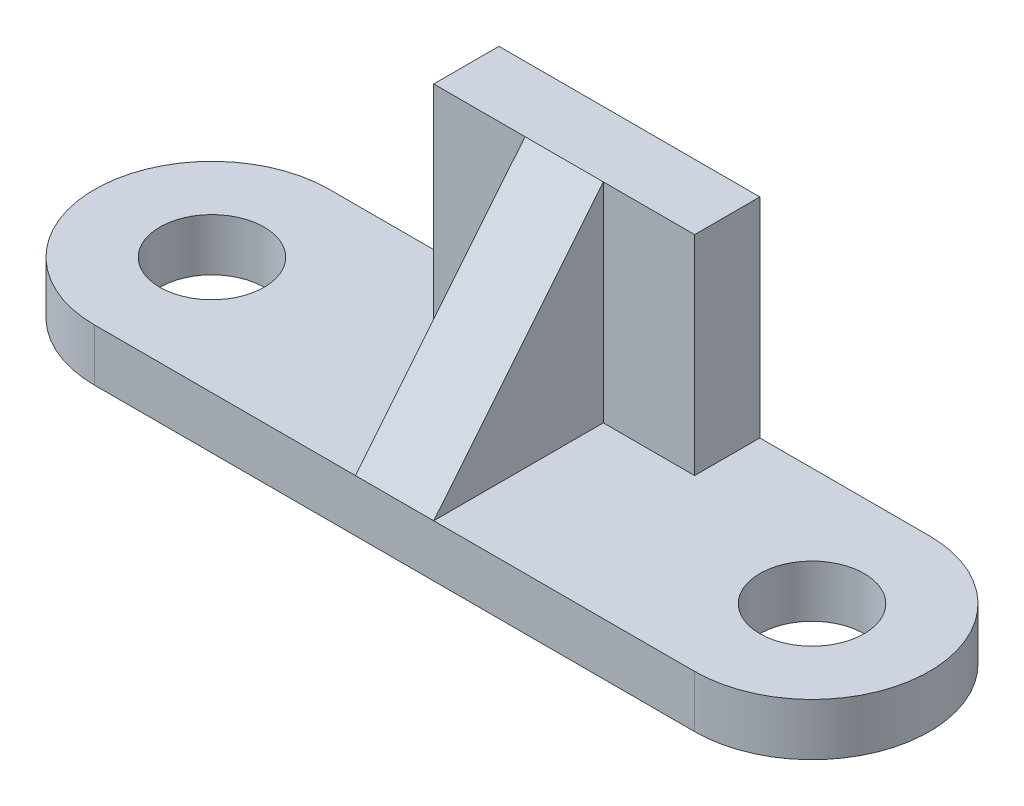
ISO-10303-21;
HEADER;
FILE_DESCRIPTION(('STEP AP214'),'2;1');
FILE_NAME('part.step','',(''),(''),'','','');
FILE_SCHEMA(('AUTOMOTIVE_DESIGN { 1 0 10303 214 1 1 1 1 }'));
ENDSEC;
DATA;
#1=APPLICATION_CONTEXT('core data for automotive mechanical design processes');
#2=APPLICATION_PROTOCOL_DEFINITION('international standard','automotive_design',2000,#1);
#3=PRODUCT_CONTEXT('',#1,'mechanical');
#4=PRODUCT('Part','Part','',(#3));
#5=PRODUCT_RELATED_PRODUCT_CATEGORY('part','',(#4));
#6=PRODUCT_DEFINITION_FORMATION('','',#4);
#7=PRODUCT_DEFINITION_CONTEXT('part definition',#1,'design');
#8=PRODUCT_DEFINITION('design','',#6,#7);
#9=PRODUCT_DEFINITION_SHAPE('','',#8);
#10=(LENGTH_UNIT() NAMED_UNIT(*) SI_UNIT(.MILLI.,.METRE.));
#11=(NAMED_UNIT(*) PLANE_ANGLE_UNIT() SI_UNIT($,.RADIAN.));
#12=(NAMED_UNIT(*) SI_UNIT($,.STERADIAN.) SOLID_ANGLE_UNIT());
#13=UNCERTAINTY_MEASURE_WITH_UNIT(LENGTH_MEASURE(1.E-05),#10,'distance_accuracy_value','');
#14=(GEOMETRIC_REPRESENTATION_CONTEXT(3) GLOBAL_UNCERTAINTY_ASSIGNED_CONTEXT((#13)) GLOBAL_UNIT_ASSIGNED_CONTEXT((#10,
#11,#12)) REPRESENTATION_CONTEXT('',''));
#15=CARTESIAN_POINT('',(0.,0.,0.));
#16=DIRECTION('',(0.,0.,1.));
#17=DIRECTION('',(1.,0.,0.));
#18=AXIS2_PLACEMENT_3D('',#15,#16,#17);
#19=CARTESIAN_POINT('',(-46.,8.,0.));
#20=DIRECTION('',(0.,1.,0.));
#21=DIRECTION('',(0.,0.,1.));
#22=AXIS2_PLACEMENT_3D('',#19,#20,#21);
#23=PLANE('',#22);
#24=CARTESIAN_POINT('',(-46.,8.,0.));
#25=DIRECTION('',(0.,1.,0.));
#26=DIRECTION('',(0.,0.,1.));
#27=AXIS2_PLACEMENT_3D('',#24,#25,#26);
#28=CIRCLE('',#27,8.);
#29=CARTESIAN_POINT('',(-46.,8.,8.));
#30=VERTEX_POINT('',#29);
#31=EDGE_CURVE('E241',#30,#30,#28,.T.);
#32=ORIENTED_EDGE('',*,*,#31,.F.);
#33=EDGE_LOOP('',(#32));
#34=FACE_BOUND('',#33,.T.);
#35=DIRECTION('',(1.,0.,0.));
#36=VECTOR('',#35,1.);
#37=CARTESIAN_POINT('',(-46.,8.,18.));
#38=LINE('',#37,#36);
#39=CARTESIAN_POINT('',(-46.,8.,18.));
#40=VERTEX_POINT('',#39);
#41=CARTESIAN_POINT('',(-6.,8.,18.));
#42=VERTEX_POINT('',#41);
#43=EDGE_CURVE('E185',#40,#42,#38,.T.);
#44=ORIENTED_EDGE('',*,*,#43,.T.);
#45=DIRECTION('',(0.,0.,-1.));
#46=VECTOR('',#45,1.);
#47=CARTESIAN_POINT('',(-6.,8.,0.));
#48=LINE('',#47,#46);
#49=CARTESIAN_POINT('',(-6.,8.,-8.));
#50=VERTEX_POINT('',#49);
#51=EDGE_CURVE('E140',#42,#50,#48,.T.);
#52=ORIENTED_EDGE('',*,*,#51,.T.);
#53=DIRECTION('',(1.,0.,0.));
#54=VECTOR('',#53,1.);
#55=CARTESIAN_POINT('',(-20.,8.,-8.));
#56=LINE('',#55,#54);
#57=CARTESIAN_POINT('',(-20.,8.,-8.));
#58=VERTEX_POINT('',#57);
#59=EDGE_CURVE('E144',#58,#50,#56,.T.);
#60=ORIENTED_EDGE('',*,*,#59,.F.);
#61=DIRECTION('',(0.,0.,1.));
#62=VECTOR('',#61,1.);
#63=CARTESIAN_POINT('',(-20.,8.,-18.));
#64=LINE('',#63,#62);
#65=CARTESIAN_POINT('',(-20.,8.,-18.));
#66=VERTEX_POINT('',#65);
#67=EDGE_CURVE('E165',#66,#58,#64,.T.);
#68=ORIENTED_EDGE('',*,*,#67,.F.);
#69=DIRECTION('',(-1.,0.,0.));
#70=VECTOR('',#69,1.);
#71=CARTESIAN_POINT('',(-46.,8.,-18.));
#72=LINE('',#71,#70);
#73=CARTESIAN_POINT('',(-46.,8.,-18.));
#74=VERTEX_POINT('',#73);
#75=EDGE_CURVE('E194',#66,#74,#72,.T.);
#76=ORIENTED_EDGE('',*,*,#75,.T.);
#77=CARTESIAN_POINT('',(-46.,8.,0.));
#78=DIRECTION('',(0.,1.,0.));
#79=DIRECTION('',(0.,0.,1.));
#80=AXIS2_PLACEMENT_3D('',#77,#78,#79);
#81=CIRCLE('',#80,18.);
#82=EDGE_CURVE('E181',#74,#40,#81,.T.);
#83=ORIENTED_EDGE('',*,*,#82,.T.);
#84=EDGE_LOOP('',(#44,#52,#60,#68,#76,#83));
#85=FACE_BOUND('',#84,.T.);
#86=ADVANCED_FACE('F39',(#34,#85),#23,.T.);
#87=CARTESIAN_POINT('',(-20.,40.,-8.));
#88=DIRECTION('',(0.,0.,-1.));
#89=DIRECTION('',(-1.,0.,0.));
#90=AXIS2_PLACEMENT_3D('',#87,#88,#89);
#91=PLANE('',#90);
#92=DIRECTION('',(0.,-1.,0.));
#93=VECTOR('',#92,1.);
#94=CARTESIAN_POINT('',(-6.,40.,-8.));
#95=LINE('',#94,#93);
#96=CARTESIAN_POINT('',(-6.,40.,-8.));
#97=VERTEX_POINT('',#96);
#98=EDGE_CURVE('E137',#97,#50,#95,.T.);
#99=ORIENTED_EDGE('',*,*,#98,.F.);
#100=DIRECTION('',(1.,0.,0.));
#101=VECTOR('',#100,1.);
#102=CARTESIAN_POINT('',(-20.,40.,-8.));
#103=LINE('',#102,#101);
#104=CARTESIAN_POINT('',(-20.,40.,-8.));
#105=VERTEX_POINT('',#104);
#106=EDGE_CURVE('E128',#105,#97,#103,.T.);
#107=ORIENTED_EDGE('',*,*,#106,.F.);
#108=DIRECTION('',(0.,-1.,0.));
#109=VECTOR('',#108,1.);
#110=CARTESIAN_POINT('',(-20.,40.,-8.));
#111=LINE('',#110,#109);
#112=EDGE_CURVE('E233',#105,#58,#111,.T.);
#113=ORIENTED_EDGE('',*,*,#112,.T.);
#114=ORIENTED_EDGE('',*,*,#59,.T.);
#115=EDGE_LOOP('',(#99,#107,#113,#114));
#116=FACE_BOUND('',#115,.T.);
#117=ADVANCED_FACE('F141',(#116),#91,.F.);
#118=CARTESIAN_POINT('',(-46.,8.,0.));
#119=DIRECTION('',(0.,-1.,0.));
#120=DIRECTION('',(0.,0.,-1.));
#121=AXIS2_PLACEMENT_3D('',#118,#119,#120);
#122=CYLINDRICAL_SURFACE('',#121,18.);
#123=CARTESIAN_POINT('',(-46.,0.,0.));
#124=DIRECTION('',(0.,1.,0.));
#125=DIRECTION('',(0.,0.,1.));
#126=AXIS2_PLACEMENT_3D('',#123,#124,#125);
#127=CIRCLE('',#126,18.);
#128=CARTESIAN_POINT('',(-46.,0.,-18.));
#129=VERTEX_POINT('',#128);
#130=CARTESIAN_POINT('',(-46.,0.,18.));
#131=VERTEX_POINT('',#130);
#132=EDGE_CURVE('E198',#129,#131,#127,.T.);
#133=ORIENTED_EDGE('',*,*,#132,.T.);
#134=DIRECTION('',(0.,-1.,0.));
#135=VECTOR('',#134,1.);
#136=CARTESIAN_POINT('',(-46.,8.,18.));
#137=LINE('',#136,#135);
#138=EDGE_CURVE('E11',#40,#131,#137,.T.);
#139=ORIENTED_EDGE('',*,*,#138,.F.);
#140=ORIENTED_EDGE('',*,*,#82,.F.);
#141=DIRECTION('',(0.,-1.,0.));
#142=VECTOR('',#141,1.);
#143=CARTESIAN_POINT('',(-46.,8.,-18.));
#144=LINE('',#143,#142);
#145=EDGE_CURVE('E193',#74,#129,#144,.T.);
#146=ORIENTED_EDGE('',*,*,#145,.T.);
#147=EDGE_LOOP('',(#133,#139,#140,#146));
#148=FACE_BOUND('',#147,.T.);
#149=ADVANCED_FACE('F41',(#148),#122,.T.);
#150=CARTESIAN_POINT('',(-46.,8.,18.));
#151=DIRECTION('',(0.,0.,-1.));
#152=DIRECTION('',(-1.,0.,0.));
#153=AXIS2_PLACEMENT_3D('',#150,#151,#152);
#154=PLANE('',#153);
#155=CARTESIAN_POINT('',(6.,8.,18.));
#156=VERTEX_POINT('',#155);
#157=CARTESIAN_POINT('',(46.,8.,18.));
#158=VERTEX_POINT('',#157);
#159=EDGE_CURVE('E171',#156,#158,#38,.T.);
#160=ORIENTED_EDGE('',*,*,#159,.F.);
#161=DIRECTION('',(1.,0.,0.));
#162=VECTOR('',#161,1.);
#163=CARTESIAN_POINT('',(-46.,8.,18.));
#164=LINE('',#163,#162);
#165=EDGE_CURVE('E159',#42,#156,#164,.T.);
#166=ORIENTED_EDGE('',*,*,#165,.F.);
#167=ORIENTED_EDGE('',*,*,#43,.F.);
#168=ORIENTED_EDGE('',*,*,#138,.T.);
#169=DIRECTION('',(1.,0.,0.));
#170=VECTOR('',#169,1.);
#171=CARTESIAN_POINT('',(-46.,0.,18.));
#172=LINE('',#171,#170);
#173=CARTESIAN_POINT('',(46.,0.,18.));
#174=VERTEX_POINT('',#173);
#175=EDGE_CURVE('E200',#131,#174,#172,.T.);
#176=ORIENTED_EDGE('',*,*,#175,.T.);
#177=DIRECTION('',(0.,-1.,0.));
#178=VECTOR('',#177,1.);
#179=CARTESIAN_POINT('',(46.,8.,18.));
#180=LINE('',#179,#178);
#181=EDGE_CURVE('E50',#158,#174,#180,.T.);
#182=ORIENTED_EDGE('',*,*,#181,.F.);
#183=EDGE_LOOP('',(#160,#166,#167,#168,#176,#182));
#184=FACE_BOUND('',#183,.T.);
#185=ADVANCED_FACE('F180',(#184),#154,.F.);
#186=CARTESIAN_POINT('',(46.,8.,0.));
#187=DIRECTION('',(0.,-1.,0.));
#188=DIRECTION('',(0.,0.,-1.));
#189=AXIS2_PLACEMENT_3D('',#186,#187,#188);
#190=CYLINDRICAL_SURFACE('',#189,18.);
#191=CARTESIAN_POINT('',(46.,0.,0.));
#192=DIRECTION('',(0.,1.,0.));
#193=DIRECTION('',(0.,0.,1.));
#194=AXIS2_PLACEMENT_3D('',#191,#192,#193);
#195=CIRCLE('',#194,18.);
#196=CARTESIAN_POINT('',(46.,0.,-18.));
#197=VERTEX_POINT('',#196);
#198=EDGE_CURVE('E205',#174,#197,#195,.T.);
#199=ORIENTED_EDGE('',*,*,#198,.T.);
#200=DIRECTION('',(0.,-1.,0.));
#201=VECTOR('',#200,1.);
#202=CARTESIAN_POINT('',(46.,8.,-18.));
#203=LINE('',#202,#201);
#204=CARTESIAN_POINT('',(46.,8.,-18.));
#205=VERTEX_POINT('',#204);
#206=EDGE_CURVE('E210',#205,#197,#203,.T.);
#207=ORIENTED_EDGE('',*,*,#206,.F.);
#208=CARTESIAN_POINT('',(46.,8.,0.));
#209=DIRECTION('',(0.,1.,0.));
#210=DIRECTION('',(0.,0.,1.));
#211=AXIS2_PLACEMENT_3D('',#208,#209,#210);
#212=CIRCLE('',#211,18.);
#213=EDGE_CURVE('E183',#158,#205,#212,.T.);
#214=ORIENTED_EDGE('',*,*,#213,.F.);
#215=ORIENTED_EDGE('',*,*,#181,.T.);
#216=EDGE_LOOP('',(#199,#207,#214,#215));
#217=FACE_BOUND('',#216,.T.);
#218=ADVANCED_FACE('F211',(#217),#190,.T.);
#219=CARTESIAN_POINT('',(-46.,8.,-18.));
#220=DIRECTION('',(0.,0.,1.));
#221=DIRECTION('',(1.,0.,0.));
#222=AXIS2_PLACEMENT_3D('',#219,#220,#221);
#223=PLANE('',#222);
#224=DIRECTION('',(-1.,0.,0.));
#225=VECTOR('',#224,1.);
#226=CARTESIAN_POINT('',(-46.,0.,-18.));
#227=LINE('',#226,#225);
#228=EDGE_CURVE('E189',#197,#129,#227,.T.);
#229=ORIENTED_EDGE('',*,*,#228,.T.);
#230=ORIENTED_EDGE('',*,*,#145,.F.);
#231=ORIENTED_EDGE('',*,*,#75,.F.);
#232=DIRECTION('',(0.,-1.,0.));
#233=VECTOR('',#232,1.);
#234=CARTESIAN_POINT('',(-20.,40.,-18.));
#235=LINE('',#234,#233);
#236=CARTESIAN_POINT('',(-20.,40.,-18.));
#237=VERTEX_POINT('',#236);
#238=EDGE_CURVE('E232',#237,#66,#235,.T.);
#239=ORIENTED_EDGE('',*,*,#238,.F.);
#240=DIRECTION('',(-1.,0.,0.));
#241=VECTOR('',#240,1.);
#242=CARTESIAN_POINT('',(20.,40.,-18.));
#243=LINE('',#242,#241);
#244=CARTESIAN_POINT('',(20.,40.,-18.));
#245=VERTEX_POINT('',#244);
#246=EDGE_CURVE('E156',#245,#237,#243,.T.);
#247=ORIENTED_EDGE('',*,*,#246,.F.);
#248=DIRECTION('',(0.,-1.,0.));
#249=VECTOR('',#248,1.);
#250=CARTESIAN_POINT('',(20.,40.,-18.));
#251=LINE('',#250,#249);
#252=CARTESIAN_POINT('',(20.,8.,-18.));
#253=VERTEX_POINT('',#252);
#254=EDGE_CURVE('E155',#245,#253,#251,.T.);
#255=ORIENTED_EDGE('',*,*,#254,.T.);
#256=EDGE_CURVE('E195',#205,#253,#72,.T.);
#257=ORIENTED_EDGE('',*,*,#256,.F.);
#258=ORIENTED_EDGE('',*,*,#206,.T.);
#259=EDGE_LOOP('',(#229,#230,#231,#239,#247,#255,#257,#258));
#260=FACE_BOUND('',#259,.T.);
#261=ADVANCED_FACE('F219',(#260),#223,.F.);
#262=DIRECTION('',(0.,0.,-1.));
#263=VECTOR('',#262,1.);
#264=CARTESIAN_POINT('',(6.,8.,0.));
#265=LINE('',#264,#263);
#266=CARTESIAN_POINT('',(6.,8.,-8.));
#267=VERTEX_POINT('',#266);
#268=EDGE_CURVE('E162',#156,#267,#265,.T.);
#269=ORIENTED_EDGE('',*,*,#268,.F.);
#270=ORIENTED_EDGE('',*,*,#159,.T.);
#271=ORIENTED_EDGE('',*,*,#213,.T.);
#272=ORIENTED_EDGE('',*,*,#256,.T.);
#273=DIRECTION('',(0.,0.,-1.));
#274=VECTOR('',#273,1.);
#275=CARTESIAN_POINT('',(20.,8.,-8.));
#276=LINE('',#275,#274);
#277=CARTESIAN_POINT('',(20.,8.,-8.));
#278=VERTEX_POINT('',#277);
#279=EDGE_CURVE('E160',#278,#253,#276,.T.);
#280=ORIENTED_EDGE('',*,*,#279,.F.);
#281=EDGE_CURVE('E64',#267,#278,#56,.T.);
#282=ORIENTED_EDGE('',*,*,#281,.F.);
#283=EDGE_LOOP('',(#269,#270,#271,#272,#280,#282));
#284=FACE_BOUND('',#283,.T.);
#285=CARTESIAN_POINT('',(46.,8.,0.));
#286=DIRECTION('',(0.,1.,0.));
#287=DIRECTION('',(0.,0.,1.));
#288=AXIS2_PLACEMENT_3D('',#285,#286,#287);
#289=CIRCLE('',#288,8.);
#290=CARTESIAN_POINT('',(46.,8.,8.));
#291=VERTEX_POINT('',#290);
#292=EDGE_CURVE('E231',#291,#291,#289,.T.);
#293=ORIENTED_EDGE('',*,*,#292,.F.);
#294=EDGE_LOOP('',(#293));
#295=FACE_BOUND('',#294,.T.);
#296=ADVANCED_FACE('F172',(#284,#295),#23,.T.);
#297=CARTESIAN_POINT('',(-46.,0.,0.));
#298=DIRECTION('',(0.,1.,0.));
#299=DIRECTION('',(0.,0.,1.));
#300=AXIS2_PLACEMENT_3D('',#297,#298,#299);
#301=PLANE('',#300);
#302=CARTESIAN_POINT('',(46.,0.,0.));
#303=DIRECTION('',(0.,1.,0.));
#304=DIRECTION('',(0.,0.,1.));
#305=AXIS2_PLACEMENT_3D('',#302,#303,#304);
#306=CIRCLE('',#305,8.);
#307=CARTESIAN_POINT('',(46.,0.,8.));
#308=VERTEX_POINT('',#307);
#309=EDGE_CURVE('E236',#308,#308,#306,.T.);
#310=ORIENTED_EDGE('',*,*,#309,.T.);
#311=EDGE_LOOP('',(#310));
#312=FACE_BOUND('',#311,.T.);
#313=ORIENTED_EDGE('',*,*,#198,.F.);
#314=ORIENTED_EDGE('',*,*,#175,.F.);
#315=ORIENTED_EDGE('',*,*,#132,.F.);
#316=ORIENTED_EDGE('',*,*,#228,.F.);
#317=EDGE_LOOP('',(#313,#314,#315,#316));
#318=FACE_BOUND('',#317,.T.);
#319=CARTESIAN_POINT('',(-46.,0.,0.));
#320=DIRECTION('',(0.,1.,0.));
#321=DIRECTION('',(0.,0.,1.));
#322=AXIS2_PLACEMENT_3D('',#319,#320,#321);
#323=CIRCLE('',#322,8.);
#324=CARTESIAN_POINT('',(-46.,0.,8.));
#325=VERTEX_POINT('',#324);
#326=EDGE_CURVE('E199',#325,#325,#323,.T.);
#327=ORIENTED_EDGE('',*,*,#326,.T.);
#328=EDGE_LOOP('',(#327));
#329=FACE_BOUND('',#328,.T.);
#330=ADVANCED_FACE('F214',(#312,#318,#329),#301,.F.);
#331=CARTESIAN_POINT('',(46.,0.,0.));
#332=DIRECTION('',(0.,1.,0.));
#333=DIRECTION('',(0.,0.,1.));
#334=AXIS2_PLACEMENT_3D('',#331,#332,#333);
#335=CYLINDRICAL_SURFACE('',#334,8.);
#336=ORIENTED_EDGE('',*,*,#309,.F.);
#337=EDGE_LOOP('',(#336));
#338=FACE_BOUND('',#337,.T.);
#339=ORIENTED_EDGE('',*,*,#292,.T.);
#340=EDGE_LOOP('',(#339));
#341=FACE_BOUND('',#340,.T.);
#342=ADVANCED_FACE('F252',(#338,#341),#335,.F.);
#343=CARTESIAN_POINT('',(-46.,0.,0.));
#344=DIRECTION('',(0.,1.,0.));
#345=DIRECTION('',(0.,0.,1.));
#346=AXIS2_PLACEMENT_3D('',#343,#344,#345);
#347=CYLINDRICAL_SURFACE('',#346,8.);
#348=ORIENTED_EDGE('',*,*,#326,.F.);
#349=EDGE_LOOP('',(#348));
#350=FACE_BOUND('',#349,.T.);
#351=ORIENTED_EDGE('',*,*,#31,.T.);
#352=EDGE_LOOP('',(#351));
#353=FACE_BOUND('',#352,.T.);
#354=ADVANCED_FACE('F254',(#350,#353),#347,.F.);
#355=CARTESIAN_POINT('',(-20.,40.,-18.));
#356=DIRECTION('',(1.,0.,0.));
#357=DIRECTION('',(0.,0.,-1.));
#358=AXIS2_PLACEMENT_3D('',#355,#356,#357);
#359=PLANE('',#358);
#360=ORIENTED_EDGE('',*,*,#67,.T.);
#361=ORIENTED_EDGE('',*,*,#112,.F.);
#362=DIRECTION('',(0.,0.,1.));
#363=VECTOR('',#362,1.);
#364=CARTESIAN_POINT('',(-20.,40.,-18.));
#365=LINE('',#364,#363);
#366=EDGE_CURVE('E149',#237,#105,#365,.T.);
#367=ORIENTED_EDGE('',*,*,#366,.F.);
#368=ORIENTED_EDGE('',*,*,#238,.T.);
#369=EDGE_LOOP('',(#360,#361,#367,#368));
#370=FACE_BOUND('',#369,.T.);
#371=ADVANCED_FACE('F235',(#370),#359,.F.);
#372=CARTESIAN_POINT('',(6.,40.,-8.));
#373=VERTEX_POINT('',#372);
#374=CARTESIAN_POINT('',(20.,40.,-8.));
#375=VERTEX_POINT('',#374);
#376=EDGE_CURVE('E133',#373,#375,#103,.T.);
#377=ORIENTED_EDGE('',*,*,#376,.F.);
#378=DIRECTION('',(0.,-1.,0.));
#379=VECTOR('',#378,1.);
#380=CARTESIAN_POINT('',(6.,40.,-8.));
#381=LINE('',#380,#379);
#382=EDGE_CURVE('E164',#373,#267,#381,.T.);
#383=ORIENTED_EDGE('',*,*,#382,.T.);
#384=ORIENTED_EDGE('',*,*,#281,.T.);
#385=DIRECTION('',(0.,-1.,0.));
#386=VECTOR('',#385,1.);
#387=CARTESIAN_POINT('',(20.,40.,-8.));
#388=LINE('',#387,#386);
#389=EDGE_CURVE('E239',#375,#278,#388,.T.);
#390=ORIENTED_EDGE('',*,*,#389,.F.);
#391=EDGE_LOOP('',(#377,#383,#384,#390));
#392=FACE_BOUND('',#391,.T.);
#393=ADVANCED_FACE('F272',(#392),#91,.F.);
#394=CARTESIAN_POINT('',(20.,40.,-8.));
#395=DIRECTION('',(-1.,0.,0.));
#396=DIRECTION('',(0.,0.,1.));
#397=AXIS2_PLACEMENT_3D('',#394,#395,#396);
#398=PLANE('',#397);
#399=ORIENTED_EDGE('',*,*,#279,.T.);
#400=ORIENTED_EDGE('',*,*,#254,.F.);
#401=DIRECTION('',(0.,0.,-1.));
#402=VECTOR('',#401,1.);
#403=CARTESIAN_POINT('',(20.,40.,-8.));
#404=LINE('',#403,#402);
#405=EDGE_CURVE('E151',#375,#245,#404,.T.);
#406=ORIENTED_EDGE('',*,*,#405,.F.);
#407=ORIENTED_EDGE('',*,*,#389,.T.);
#408=EDGE_LOOP('',(#399,#400,#406,#407));
#409=FACE_BOUND('',#408,.T.);
#410=ADVANCED_FACE('F287',(#409),#398,.F.);
#411=CARTESIAN_POINT('',(0.,40.,0.));
#412=DIRECTION('',(0.,1.,0.));
#413=DIRECTION('',(0.,0.,1.));
#414=AXIS2_PLACEMENT_3D('',#411,#412,#413);
#415=PLANE('',#414);
#416=ORIENTED_EDGE('',*,*,#246,.T.);
#417=ORIENTED_EDGE('',*,*,#366,.T.);
#418=ORIENTED_EDGE('',*,*,#106,.T.);
#419=EDGE_CURVE('E125',#97,#373,#103,.T.);
#420=ORIENTED_EDGE('',*,*,#419,.T.);
#421=ORIENTED_EDGE('',*,*,#376,.T.);
#422=ORIENTED_EDGE('',*,*,#405,.T.);
#423=EDGE_LOOP('',(#416,#417,#418,#420,#421,#422));
#424=FACE_BOUND('',#423,.T.);
#425=ADVANCED_FACE('F150',(#424),#415,.T.);
#426=CARTESIAN_POINT('',(0.,40.,-8.));
#427=DIRECTION('',(0.,0.630592625094466,0.776114000116266));
#428=DIRECTION('',(0.,-0.776114000116265,0.630592625094466));
#429=AXIS2_PLACEMENT_3D('',#426,#427,#428);
#430=PLANE('',#429);
#431=DIRECTION('',(0.,-0.776114000116265,0.630592625094466));
#432=VECTOR('',#431,1.);
#433=CARTESIAN_POINT('',(-6.,40.,-8.));
#434=LINE('',#433,#432);
#435=EDGE_CURVE('E127',#97,#42,#434,.T.);
#436=ORIENTED_EDGE('',*,*,#435,.T.);
#437=ORIENTED_EDGE('',*,*,#165,.T.);
#438=DIRECTION('',(0.,-0.776114000116265,0.630592625094466));
#439=VECTOR('',#438,1.);
#440=CARTESIAN_POINT('',(6.,40.,-8.));
#441=LINE('',#440,#439);
#442=EDGE_CURVE('E53',#373,#156,#441,.T.);
#443=ORIENTED_EDGE('',*,*,#442,.F.);
#444=ORIENTED_EDGE('',*,*,#419,.F.);
#445=EDGE_LOOP('',(#436,#437,#443,#444));
#446=FACE_BOUND('',#445,.T.);
#447=ADVANCED_FACE('F123',(#446),#430,.T.);
#448=CARTESIAN_POINT('',(6.,20.,0.));
#449=DIRECTION('',(1.,0.,0.));
#450=DIRECTION('',(0.,0.,-1.));
#451=AXIS2_PLACEMENT_3D('',#448,#449,#450);
#452=PLANE('',#451);
#453=ORIENTED_EDGE('',*,*,#442,.T.);
#454=ORIENTED_EDGE('',*,*,#268,.T.);
#455=ORIENTED_EDGE('',*,*,#382,.F.);
#456=EDGE_LOOP('',(#453,#454,#455));
#457=FACE_BOUND('',#456,.T.);
#458=ADVANCED_FACE('F168',(#457),#452,.T.);
#459=CARTESIAN_POINT('',(-6.,20.,0.));
#460=DIRECTION('',(1.,0.,0.));
#461=DIRECTION('',(0.,0.,-1.));
#462=AXIS2_PLACEMENT_3D('',#459,#460,#461);
#463=PLANE('',#462);
#464=ORIENTED_EDGE('',*,*,#51,.F.);
#465=ORIENTED_EDGE('',*,*,#435,.F.);
#466=ORIENTED_EDGE('',*,*,#98,.T.);
#467=EDGE_LOOP('',(#464,#465,#466));
#468=FACE_BOUND('',#467,.T.);
#469=ADVANCED_FACE('F131',(#468),#463,.F.);
#470=CLOSED_SHELL('',(#86,#117,#149,#185,#218,#261,#296,#330,#342,#354,#371,#393,#410,#425,#447,
#458,#469));
#471=MANIFOLD_SOLID_BREP('B2',#470);
#472=ADVANCED_BREP_SHAPE_REPRESENTATION('',(#18,#471),#14);
#473=SHAPE_DEFINITION_REPRESENTATION(#9,#472);
ENDSEC;
END-ISO-10303-21;
